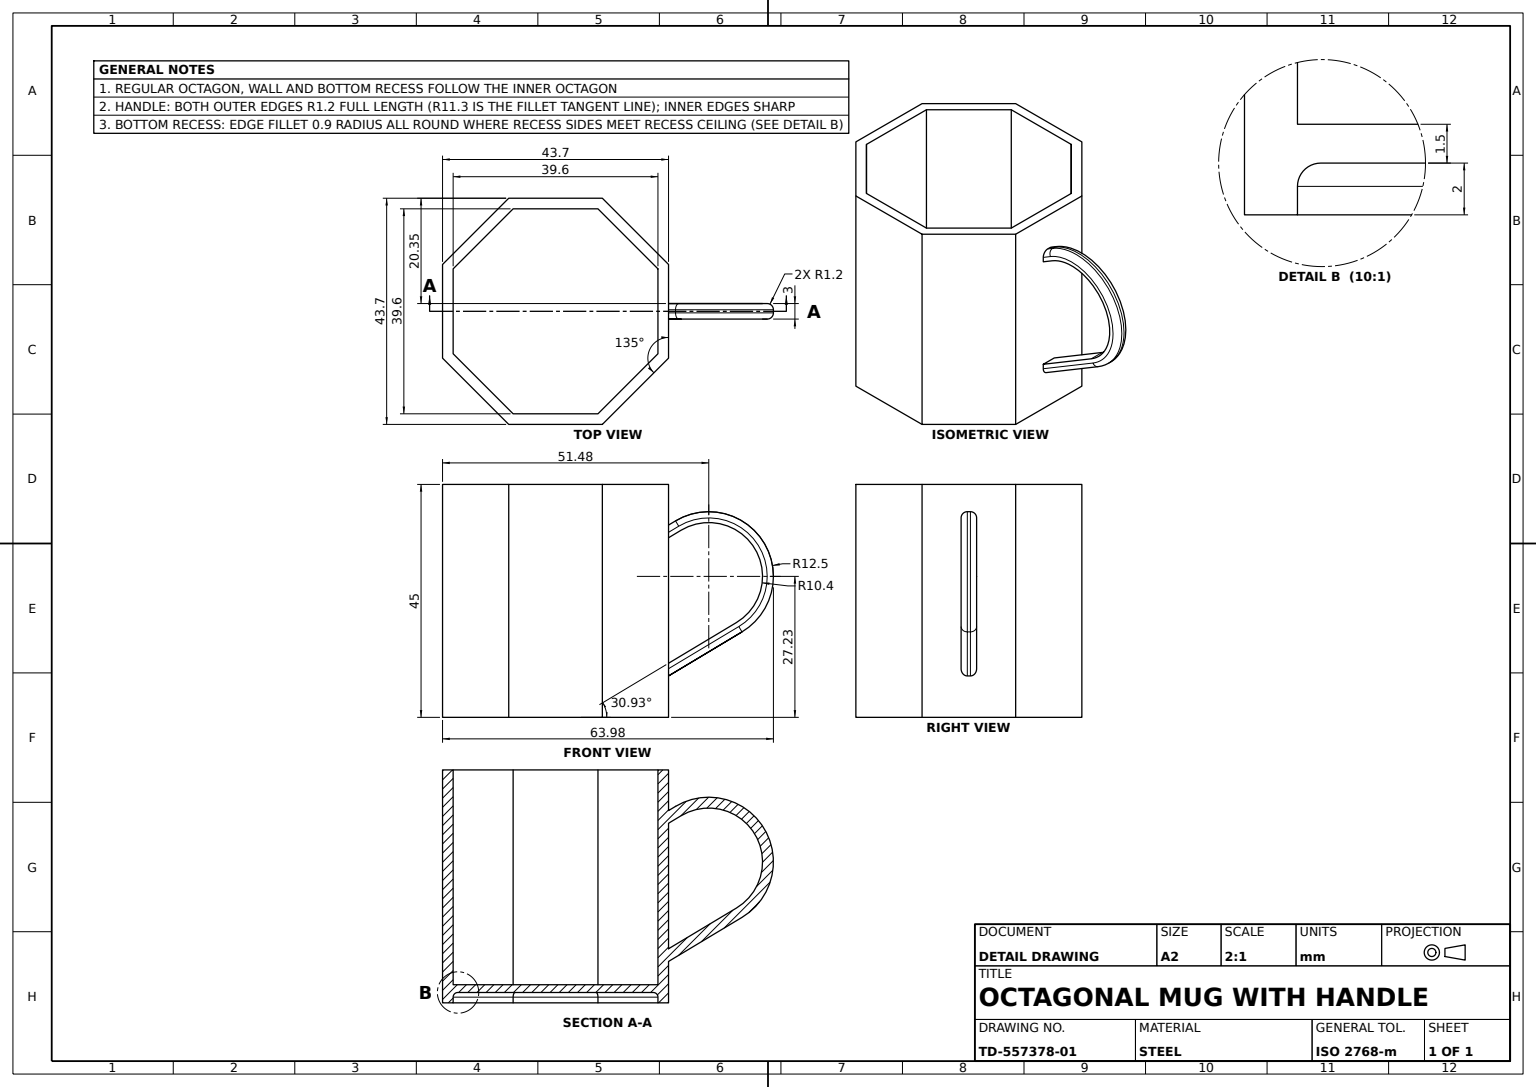
SolidWorks part; units mm, degrees
material "Plain Carbon Steel"
ref_plane "Front Plane" through (0, 0, 0) normal (0, 0, 1) x (1, 0, 0)
ref_plane "Top Plane" through (0, 0, 0) normal (0, 1, 0) x (1, 0, 0)
ref_plane "Right Plane" through (0, 0, 0) normal (1, 0, 0) x (0, 0, -1)
sketch "Wall Profile Octagon" plane through (0, 0, 0) normal (0, 1, 0) x (1, 0, 0)
  line L1 (21.8486, -9.05) -> (21.8486, 9.05)
  line L2 (21.8486, 9.05) -> (9.05, 21.8486)
  line L3 (9.05, 21.8486) -> (-9.05, 21.8486)
  line L4 (-9.05, 21.8486) -> (-21.8486, 9.05)
  line L5 (-21.8486, 9.05) -> (-21.8486, -9.05)
  line L6 (-21.8486, -9.05) -> (-9.05, -21.8486)
  line L7 (-9.05, -21.8486) -> (9.05, -21.8486)
  line L8 (9.05, -21.8486) -> (21.8486, -9.05)
  line L9 (19.8, 8.2014) -> (8.2014, 19.8)
  line L10 (8.2014, 19.8) -> (-8.2014, 19.8)
  line L11 (-8.2014, 19.8) -> (-19.8, 8.2014)
  line L12 (-19.8, 8.2014) -> (-19.8, -8.2014)
  line L13 (-19.8, -8.2014) -> (-8.2014, -19.8)
  line L14 (-8.2014, -19.8) -> (8.2014, -19.8)
  line L15 (8.2014, -19.8) -> (19.8, -8.2014)
  line L16 (19.8, -8.2014) -> (19.8, 8.2014)
  circle A0 centre (0, 0) radius 21.8486 construction
  circle A1 centre (0, 0) radius 19.8 construction
  dimension "D2" = 39.6
  dimension "D1" = 18.1
extrude "Mug Wall" add sketch "Wall Profile Octagon" along normal mid plane 45
ref_plane "Bottom Offset Plane" through (0, -20.5, 0) normal (0, 1, 0) x (1, 0, 0)
sketch "Bottom Profile Octagon" plane through (0, -20.5, 0) normal (0, 1, 0) x (1, 0, 0)
  line L0 (-19.8, 8.2014) -> (-19.8, -8.2014) construction
  line L1 (-19.8, -8.2014) -> (-8.2014, -19.8) construction
  line L2 (-8.2014, -19.8) -> (8.2014, -19.8) construction
  line L3 (8.2014, -19.8) -> (19.8, -8.2014) construction
  line L4 (19.8, -8.2014) -> (19.8, 8.2014) construction
  line L5 (19.8, 8.2014) -> (8.2014, 19.8) construction
  line L6 (8.2014, 19.8) -> (-8.2014, 19.8) construction
  line L7 (-8.2014, 19.8) -> (-19.8, 8.2014) construction
  line L8 (-19.8, 8.2014) -> (-19.8, -8.2014)
  line L9 (-19.8, -8.2014) -> (-8.2014, -19.8)
  line L10 (-8.2014, -19.8) -> (8.2014, -19.8)
  line L11 (8.2014, -19.8) -> (19.8, -8.2014)
  line L12 (19.8, -8.2014) -> (19.8, 8.2014)
  line L13 (19.8, 8.2014) -> (8.2014, 19.8)
  line L14 (8.2014, 19.8) -> (-8.2014, 19.8)
  line L15 (-8.2014, 19.8) -> (-19.8, 8.2014)
extrude "Mug Bottom" add sketch "Bottom Profile Octagon" along normal blind 1.5
fillet "Bottom Edge Fillet R0.9" radius 0.9 8 edges at (-19.8, -20.5, 0) (-14.0007, -20.5, 14.0007) (0, -20.5, 19.8) (14.0007, -20.5, 14.0007) (19.8, -20.5, 0) (14.0007, -20.5, -14.0007) (0, -20.5, -19.8) (-14.0007, -20.5, -14.0007)
sketch "Handle Profile" plane through (0, 0, 0) normal (0, 0, 1) x (1, 0, 0)
  line L0 (21.8486, -12.0519) -> (34.973, -4.1879)
  line L1 (21.8486, 22.5) -> (21.8486, -22.5) construction
  line L2 (24.2821, 13.6543) -> (21.8486, 12.1962)
  line L3 (21.8486, -14.5) -> (36.0523, -5.9893)
  line L4 (23.2027, 15.4557) -> (21.8486, 14.6443)
  line L5 (9.05, -22.5) -> (21.8486, -22.5) construction
  line L6 (21.8486, 12.1962) -> (21.8486, 14.6443)
  line L7 (21.8486, -14.5) -> (21.8486, -12.0519)
  arc A0 (34.973, -4.1879) -> (24.2821, 13.6543) centre (29.6275, 4.7332) ccw
  arc A1 (36.0523, -5.9893) -> (23.2027, 15.4557) centre (29.6275, 4.7332) ccw
  point P6 (38.5486, 10.0786)
  dimension "D4" = 12.5
  dimension "D5" = 10.4
  dimension "D1" = 15.3
  dimension "D2" = 20.8
  dimension "D3" = 16.7
  dimension "D6" = 8
extrude "Handle" add sketch "Handle Profile" along normal mid plane 3
fillet "Handle Edge Fillet R1.2" radius 1.2 6 edges at (28.9505, -10.2446, 1.5) (22.5257, 15.05, 1.5) (28.9505, -10.2446, -1.5) (22.5257, 15.05, -1.5) (40.35, 11.158, 1.5) (40.35, 11.158, -1.5)
